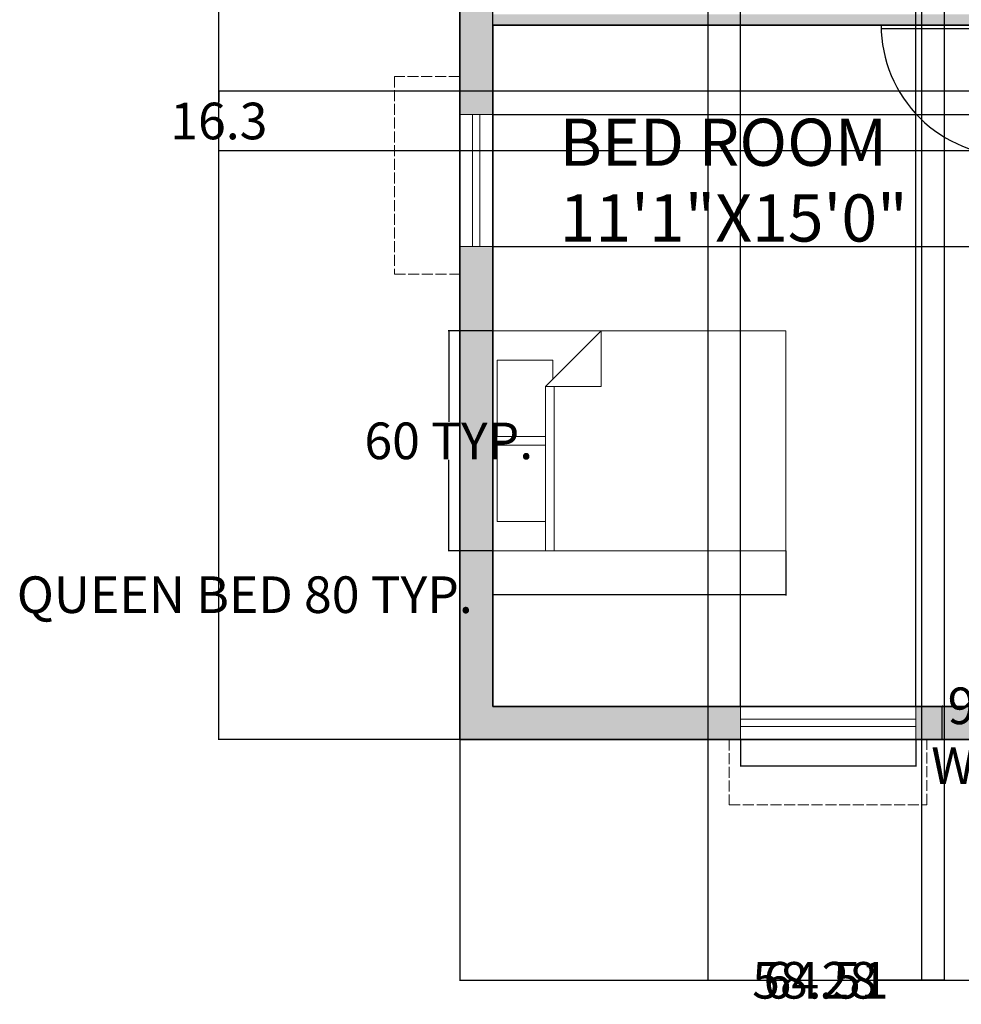
# Model space of a CAD drawing. Units: inches. Extents: x 300 to 1007, y 2 to 1069.
# Tile 1 of 12: x 300 to 557, y 2 to 271. Entities that reach past the tile are written whole.
import ezdxf

# ---------------------------------------------------------------- set-up
doc = ezdxf.new("R2010")
doc.units = ezdxf.units.IN
doc.header["$MEASUREMENT"] = 0
doc.linetypes.add('ACAD_ISO02W100', pattern=[15, 12, -3])
for name, color, linetype, lineweight in [('A-ANNO-DIMS', 2, 'Continuous', 18), ('A-AREA-IDEN', 7, 'Continuous', 18), ('A-DOOR', 3, 'Continuous', 25), ('A-FURN', 8, 'Continuous', 18), ('A-GLAZ', 4, 'Continuous', 18), ('A-GLAZ-OVHD', 8, 'ACAD_ISO02W100', 13), ('A-WALL', 7, 'Continuous', 35)]:
    doc.layers.add(name, color=color, linetype=linetype, lineweight=lineweight)
doc.layers.add('A-WALL-PATT', color=9, linetype='Continuous', lineweight=9, true_color=0xc7c8ca)
doc.styles.get("Standard").update_dxf_attribs({"font": 'arial.ttf'})
doc.dimstyles.get("Standard").update_dxf_attribs({"dimtxt": 10, "dimasz": 0.18, "dimexe": 0.18, "dimexo": 0.0625, "dimgap": 0.09, "dimtad": 0, "dimtih": 1, "dimtoh": 1, "dimdec": 0, "dimzin": 0, "dimdsep": 46, "dimlunit": 3, "dimtxsty": 'Standard', "dimcen": 0.09, "dimadec": 0, "dimazin": 0, "dimtfac": 1, "dimtdec": 0, "dimtofl": 0, "dimtmove": 0, "dimatfit": 3, "dimfxl": 1, "dimtolj": 1, "dimtzin": 0, "dimarcsym": 0})

# ---------------------------------------------------------------- blocks, each defined once
blk = doc.blocks.new('Bed - Queen')
for p, q in [((0, -80.00003), (0, 0)), ((0, 0), (59.99999, 0)), ((59.99999, 0), (59.99999, -80.00003)), ((7.99999, -1.2), (28.79998, -1.2)), ((7.99999, -14.4), (7.99999, -1.2)), ((28.79998, -1.2), (28.79998, -14.4)), ((31.19999, -1.2), (51.99999, -1.2)), ((31.19999, -14.4), (31.19999, -1.2)), ((51.99999, -1.2), (51.99999, -16.4)), ((0, -14.4), (44.8, -14.4)), ((59.99999, -29.6), (44.8, -14.4)), ((44.8, -14.4), (44.8, -29.6)), ((44.8, -16.8), (0, -16.8)), ((51.99999, -16.4), (46.79936, -16.4)), ((44.8, -29.6), (59.99999, -29.6)), ((59.99999, -80.00003), (0, -80.00003))]:
    blk.add_line(p, q)
blk = doc.blocks.new('WIN-48')
for p, q in [((-47.83, 0), (-47.83, 4.5)), ((-47.83, 4.5), (-47.83, -4.5)), ((0, 4.5), (0, -4.5)), ((0, 1), (-47.83, 1)), ((0, -1), (-47.83, -1))]:
    blk.add_line(p, q)
blk = doc.blocks.new('WIN-36')
for p, q in [((-36, -4.5), (-36, 4.5)), ((0, -4.5), (0, 4.5)), ((0, 1), (-36, 1)), ((-36, 0), (-36, -4.5)), ((0, -1), (-36, -1))]:
    blk.add_line(p, q)
blk = doc.blocks.new('WINDOW-HOOD-54')
at = {"ltscale": 0.25}
for p, q in [((0, 17.83), (-53.97, 17.83)), ((-53.97, 17.83), (-53.97, 0)), ((0, 0), (0, 17.83))]:
    blk.add_line(p, q, dxfattribs=at)
blk = doc.blocks.new('DOOR-SINGLE-36')
for p, q in [((-1, 0), (-1, 36)), ((0, 0), (0, 36))]:
    blk.add_line(p, q)
blk.add_arc((0, 0.34), 35.66, 90, 180.5503)
blk = doc.blocks.new('*D29')
at = {"layer": 'A-ANNO-DIMS', "color": 0, "lineweight": -2, "transparency": 16777216}
for p, q in [((429.12, 125.84), (429.12, 113.72)), ((509.12, 125.84), (509.12, 113.72)), ((429.12, 113.9), (428.94, 113.9)), ((508.94, 113.9), (429.3, 113.9))]:
    blk.add_line(p, q, dxfattribs=at)
at = {"layer": 'A-ANNO-DIMS', "color": 0, "transparency": 16777216}
for points in [[(429.3, 113.93), (429.3, 113.87), (429.12, 113.9)], [(508.94, 113.93), (508.94, 113.87), (509.12, 113.9)]]:
    blk.add_solid(points, dxfattribs=at)
at = {"layer": 'Defpoints', "color": 0, "transparency": 16777216}
for p in [(429.12, 125.9), (509.12, 125.9), (429.12, 113.9)]:
    blk.add_point(p, dxfattribs=at)
at = {"layer": 'A-ANNO-DIMS', "color": 0, "transparency": 16777216, "insert": (361.44, 113.9), "char_height": 10, "attachment_point": 5}
blk.add_mtext('\\A1;QUEEN BED 80 TYP.', dxfattribs=at)
blk = doc.blocks.new('*D30')
at = {"layer": 'A-ANNO-DIMS', "color": 0, "lineweight": -2, "transparency": 16777216}
for p, q in [((429.06, 185.9), (416.94, 185.9)), ((417.12, 185.72), (417.12, 161.09)), ((417.12, 126.08), (417.12, 150.7)), ((429.06, 125.9), (416.94, 125.9))]:
    blk.add_line(p, q, dxfattribs=at)
at = {"layer": 'A-ANNO-DIMS', "color": 0, "transparency": 16777216}
for points in [[(417.09, 185.72), (417.15, 185.72), (417.12, 185.9)], [(417.09, 126.08), (417.15, 126.08), (417.12, 125.9)]]:
    blk.add_solid(points, dxfattribs=at)
at = {"layer": 'Defpoints', "color": 0, "transparency": 16777216}
for p in [(417.12, 185.9), (429.12, 185.9), (429.12, 125.9)]:
    blk.add_point(p, dxfattribs=at)
at = {"layer": 'A-ANNO-DIMS', "color": 0, "transparency": 16777216, "insert": (417.12, 155.9), "char_height": 10, "attachment_point": 5}
blk.add_mtext('\\A1;60 TYP.', dxfattribs=at)
blk = doc.blocks.new('*D43')
at = {"layer": 'A-ANNO-DIMS', "color": 0, "lineweight": -2, "transparency": 16777216}
for p, q in [((496.77, 74.32), (496.77, 67.03)), ((544.6, 74.32), (544.6, 67.03)), ((496.95, 67.21), (544.42, 67.21)), ((544.6, 67.21), (544.78, 67.21))]:
    blk.add_line(p, q, dxfattribs=at)
at = {"layer": 'A-ANNO-DIMS', "color": 0, "transparency": 16777216}
for points in [[(496.95, 67.24), (496.95, 67.18), (496.77, 67.21)], [(544.42, 67.24), (544.42, 67.18), (544.6, 67.21)]]:
    blk.add_solid(points, dxfattribs=at)
at = {"layer": 'Defpoints', "color": 0, "transparency": 16777216}
for p in [(496.77, 74.38), (544.6, 74.38), (544.6, 67.21)]:
    blk.add_point(p, dxfattribs=at)
at = {"layer": 'A-ANNO-DIMS', "color": 0, "transparency": 16777216, "insert": (602, 67.21), "char_height": 10, "attachment_point": 5}
blk.add_mtext('\\A1;WINDOW 48 TYP.', dxfattribs=at)
blk = doc.blocks.new('*D44')
at = {"layer": 'A-ANNO-DIMS', "color": 0, "lineweight": -2, "transparency": 16777216}
for p, q in [((544.67, 83.38), (551.96, 83.38)), ((551.78, 83.38), (551.78, 83.56)), ((551.78, 83.56), (551.96, 83.56)), ((551.78, 74.56), (551.78, 83.2)), ((544.67, 74.38), (551.96, 74.38))]:
    blk.add_line(p, q, dxfattribs=at)
at = {"layer": 'A-ANNO-DIMS', "color": 0, "transparency": 16777216}
for points in [[(551.75, 83.2), (551.81, 83.2), (551.78, 83.38)], [(551.75, 74.56), (551.81, 74.56), (551.78, 74.38)]]:
    blk.add_solid(points, dxfattribs=at)
at = {"layer": 'Defpoints', "color": 0, "transparency": 16777216}
for p in [(544.6, 83.38), (551.78, 83.38), (544.6, 74.38)]:
    blk.add_point(p, dxfattribs=at)
at = {"layer": 'A-ANNO-DIMS', "color": 0, "transparency": 16777216, "insert": (572.5, 83.56), "char_height": 10, "attachment_point": 5}
blk.add_mtext('\\A1;9 TYP.', dxfattribs=at)
blk = doc.blocks.new('*D73')
at = {"layer": 'A-ANNO-DIMS', "color": 0, "lineweight": -2, "transparency": 16777216}
for p, q in [((420.12, 74.32), (420.12, 8.45)), ((910.12, 74.32), (910.12, 8.45)), ((420.3, 8.63), (653.8, 8.63)), ((909.94, 8.63), (676.44, 8.63))]:
    blk.add_line(p, q, dxfattribs=at)
at = {"layer": 'A-ANNO-DIMS', "color": 0, "transparency": 16777216}
for points in [[(420.3, 8.66), (420.3, 8.6), (420.12, 8.63)], [(909.94, 8.66), (909.94, 8.6), (910.12, 8.63)]]:
    blk.add_solid(points, dxfattribs=at)
at = {"layer": 'Defpoints', "color": 0, "transparency": 16777216}
for p in [(420.12, 74.38), (910.12, 74.38), (910.12, 8.63)]:
    blk.add_point(p, dxfattribs=at)
at = {"layer": 'A-ANNO-DIMS', "color": 0, "transparency": 16777216, "insert": (665.12, 8.63), "char_height": 10, "attachment_point": 5}
blk.add_mtext('\\A1;490', dxfattribs=at)
blk = doc.blocks.new('*D74')
at = {"layer": 'A-ANNO-DIMS', "color": 0, "lineweight": -2, "transparency": 16777216}
for p, q in [((478.76, 999.45), (354.19, 999.45)), ((354.37, 999.27), (354.37, 542.11)), ((354.37, 74.56), (354.37, 531.72)), ((420.06, 74.38), (354.19, 74.38))]:
    blk.add_line(p, q, dxfattribs=at)
at = {"layer": 'A-ANNO-DIMS', "color": 0, "transparency": 16777216}
for points in [[(354.34, 999.27), (354.4, 999.27), (354.37, 999.45)], [(354.34, 74.56), (354.4, 74.56), (354.37, 74.38)]]:
    blk.add_solid(points, dxfattribs=at)
at = {"layer": 'Defpoints', "color": 0, "transparency": 16777216}
for p in [(354.37, 999.45), (478.83, 999.45), (420.12, 74.38)]:
    blk.add_point(p, dxfattribs=at)
at = {"layer": 'A-ANNO-DIMS', "color": 0, "transparency": 16777216, "insert": (354.37, 536.92), "char_height": 10, "attachment_point": 5}
blk.add_mtext('\\A1;925', dxfattribs=at)
blk = doc.blocks.new('*D87')
at = {"layer": 'A-ANNO-DIMS', "color": 0, "lineweight": -2, "transparency": 16777216}
for p, q in [((805.89, 251.38), (354.19, 251.38)), ((354.37, 251.2), (354.37, 248.43)), ((354.37, 235.26), (354.37, 238.03)), ((805.89, 235.08), (354.19, 235.08))]:
    blk.add_line(p, q, dxfattribs=at)
at = {"layer": 'A-ANNO-DIMS', "color": 0, "transparency": 16777216}
for points in [[(354.34, 251.2), (354.4, 251.2), (354.37, 251.38)], [(354.34, 235.26), (354.4, 235.26), (354.37, 235.08)]]:
    blk.add_solid(points, dxfattribs=at)
at = {"layer": 'Defpoints', "color": 0, "transparency": 16777216}
for p in [(805.95, 251.38), (354.37, 235.08), (805.95, 235.08)]:
    blk.add_point(p, dxfattribs=at)
at = {"layer": 'A-ANNO-DIMS', "color": 0, "transparency": 16777216, "insert": (354.37, 243.23), "char_height": 10, "attachment_point": 5}
blk.add_mtext('\\A1;16.3', dxfattribs=at)
blk = doc.blocks.new('*D88')
at = {"layer": 'A-ANNO-DIMS', "color": 0, "lineweight": -2, "transparency": 16777216}
for p, q in [((429.12, 83.45), (429.12, 1063.03)), ((429.3, 1062.85), (445.92, 1062.85)), ((496.59, 1062.85), (479.97, 1062.85)), ((496.77, 83.45), (496.77, 1063.03))]:
    blk.add_line(p, q, dxfattribs=at)
at = {"layer": 'A-ANNO-DIMS', "color": 0, "transparency": 16777216}
for points in [[(429.3, 1062.88), (429.3, 1062.82), (429.12, 1062.85)], [(496.59, 1062.88), (496.59, 1062.82), (496.77, 1062.85)]]:
    blk.add_solid(points, dxfattribs=at)
at = {"layer": 'Defpoints', "color": 0, "transparency": 16777216}
for p in [(496.77, 1062.85), (429.12, 83.38), (496.77, 83.38)]:
    blk.add_point(p, dxfattribs=at)
at = {"layer": 'A-ANNO-DIMS', "color": 0, "transparency": 16777216, "insert": (462.95, 1062.85), "char_height": 10, "attachment_point": 5}
blk.add_mtext('\\A1;67.65', dxfattribs=at)
blk = doc.blocks.new('*D89')
at = {"layer": 'A-ANNO-DIMS', "color": 0, "lineweight": -2, "transparency": 16777216}
for p, q in [((544.6, 83.45), (544.6, 1063.03)), ((544.78, 1062.85), (554.56, 1062.85)), ((598.25, 1062.85), (588.48, 1062.85)), ((598.43, 83.45), (598.43, 1063.03))]:
    blk.add_line(p, q, dxfattribs=at)
at = {"layer": 'A-ANNO-DIMS', "color": 0, "transparency": 16777216}
for points in [[(544.78, 1062.88), (544.78, 1062.82), (544.6, 1062.85)], [(598.25, 1062.88), (598.25, 1062.82), (598.43, 1062.85)]]:
    blk.add_solid(points, dxfattribs=at)
at = {"layer": 'Defpoints', "color": 0, "transparency": 16777216}
for p in [(598.43, 1062.85), (544.6, 83.38), (598.43, 83.38)]:
    blk.add_point(p, dxfattribs=at)
at = {"layer": 'A-ANNO-DIMS', "color": 0, "transparency": 16777216, "insert": (571.52, 1062.85), "char_height": 10, "attachment_point": 5}
blk.add_mtext('\\A1;53.83', dxfattribs=at)
blk = doc.blocks.new('*D90')
at = {"layer": 'A-ANNO-DIMS', "color": 0, "lineweight": -2, "transparency": 16777216}
for p, q in [((429.18, 209), (974.48, 209)), ((974.3, 208.82), (974.3, 151.39)), ((974.3, 83.56), (974.3, 141)), ((429.18, 83.38), (974.48, 83.38))]:
    blk.add_line(p, q, dxfattribs=at)
at = {"layer": 'A-ANNO-DIMS', "color": 0, "transparency": 16777216}
for points in [[(974.27, 208.82), (974.33, 208.82), (974.3, 209)], [(974.27, 83.56), (974.33, 83.56), (974.3, 83.38)]]:
    blk.add_solid(points, dxfattribs=at)
at = {"layer": 'Defpoints', "color": 0, "transparency": 16777216}
for p in [(429.12, 209), (974.3, 209), (429.12, 83.38)]:
    blk.add_point(p, dxfattribs=at)
at = {"layer": 'A-ANNO-DIMS', "color": 0, "transparency": 16777216, "insert": (974.3, 146.19), "char_height": 10, "attachment_point": 5}
blk.add_mtext('\\A1;125.61', dxfattribs=at)
blk = doc.blocks.new('*D91')
at = {"layer": 'A-ANNO-DIMS', "color": 0, "lineweight": -2, "transparency": 16777216}
for p, q in [((429.18, 325.09), (974.48, 325.09)), ((974.3, 324.91), (974.3, 290.23)), ((974.3, 245.16), (974.3, 279.84)), ((429.18, 244.98), (974.48, 244.98))]:
    blk.add_line(p, q, dxfattribs=at)
at = {"layer": 'A-ANNO-DIMS', "color": 0, "transparency": 16777216}
for points in [[(974.27, 324.91), (974.33, 324.91), (974.3, 325.09)], [(974.27, 245.16), (974.33, 245.16), (974.3, 244.98)]]:
    blk.add_solid(points, dxfattribs=at)
at = {"layer": 'Defpoints', "color": 0, "transparency": 16777216}
for p in [(429.12, 325.09), (974.3, 325.09), (429.12, 244.98)]:
    blk.add_point(p, dxfattribs=at)
at = {"layer": 'A-ANNO-DIMS', "color": 0, "transparency": 16777216, "insert": (974.3, 285.04), "char_height": 10, "attachment_point": 5}
blk.add_mtext('\\A1;80.11', dxfattribs=at)
blk = doc.blocks.new('*D101')
at = {"layer": 'A-ANNO-DIMS', "color": 0, "lineweight": -2, "transparency": 16777216}
for p, q in [((487.83, 609.38), (487.83, 8.45)), ((552.34, 609.38), (552.34, 8.45)), ((488.01, 8.63), (504.06, 8.63)), ((552.16, 8.63), (536.11, 8.63))]:
    blk.add_line(p, q, dxfattribs=at)
at = {"layer": 'A-ANNO-DIMS', "color": 0, "transparency": 16777216}
for points in [[(488.01, 8.66), (488.01, 8.6), (487.83, 8.63)], [(552.16, 8.66), (552.16, 8.6), (552.34, 8.63)]]:
    blk.add_solid(points, dxfattribs=at)
at = {"layer": 'Defpoints', "color": 0, "transparency": 16777216}
for p in [(487.83, 609.45), (552.34, 609.45), (552.34, 8.63)]:
    blk.add_point(p, dxfattribs=at)
at = {"layer": 'A-ANNO-DIMS', "color": 0, "transparency": 16777216, "insert": (520.08, 8.63), "char_height": 10, "attachment_point": 5}
blk.add_mtext('\\A1;64.51', dxfattribs=at)
blk = doc.blocks.new('*D105')
at = {"layer": 'A-ANNO-DIMS', "color": 0, "lineweight": -2, "transparency": 16777216}
for p, q in [((487.83, 990.38), (487.83, 8.45)), ((546.1, 990.38), (546.1, 8.45)), ((488.01, 8.63), (499.99, 8.63)), ((545.92, 8.63), (533.94, 8.63))]:
    blk.add_line(p, q, dxfattribs=at)
at = {"layer": 'A-ANNO-DIMS', "color": 0, "transparency": 16777216}
for points in [[(488.01, 8.66), (488.01, 8.6), (487.83, 8.63)], [(545.92, 8.66), (545.92, 8.6), (546.1, 8.63)]]:
    blk.add_solid(points, dxfattribs=at)
at = {"layer": 'Defpoints', "color": 0, "transparency": 16777216}
for p in [(487.83, 990.45), (546.1, 990.45), (546.1, 8.63)]:
    blk.add_point(p, dxfattribs=at)
at = {"layer": 'A-ANNO-DIMS', "color": 0, "transparency": 16777216, "insert": (516.97, 8.63), "char_height": 10, "attachment_point": 5}
blk.add_mtext('\\A1;58.28', dxfattribs=at)

msp = doc.modelspace()

# ---------------------------------------------------------------- hatches: boundary and pattern name
at = {"layer": 'A-WALL-PATT'}
h = msp.add_hatch(color=256, dxfattribs=at)
h.dxf.hatch_style = 1
h.paths.add_polyline_path([(546.104, 999.4468), (478.8267, 999.4468), (478.8267, 869.2798, -0.06322715), (487.8267, 868.1328), (487.8267, 990.4468), (546.104, 990.4468)])
h.paths.add_polyline_path([(630.4852, 999.4468), (582.106, 999.4468), (582.106, 990.4468), (613.8267, 990.4468), (613.8267, 867.4468), (622.8267, 867.4468), (622.8267, 990.4468), (630.4852, 990.4468)])
h.paths.add_polyline_path([(702.0883, 999.4468), (650.4653, 999.4468), (650.4653, 990.4468), (682.8267, 990.4468), (682.8267, 960.0824, -0.02530575), (685.8267, 960.0478), (685.8267, 990.4468), (702.0883, 990.4468)])
h.paths.add_polyline_path([(850.8267, 999.4468), (737.5888, 999.4468), (737.5888, 990.4468), (841.8267, 990.4468), (841.8267, 950.5685), (850.8267, 950.5685)])
h.paths.add_polyline_path([(685.8267, 930.4465), (682.8267, 930.4465), (682.8267, 888.4468), (682.8267, 867.4468), (685.8267, 867.4468), (697.4169, 867.4468), (697.4169, 870.4468), (685.8267, 870.4468), (685.8267, 888.4468)])
h.paths.add_polyline_path([(682.8267, 931.4465), (654.3436, 931.4465, 0.00843109), (654.3267, 930.4465), (682.8267, 930.4465)])
h.paths.add_polyline_path([(685.8267, 931.4465), (682.8267, 931.4465), (682.8267, 930.4465), (685.8267, 930.4465)])
h.paths.add_polyline_path([(682.8267, 888.4468), (622.8267, 888.4468), (622.8267, 885.4468), (682.8267, 885.4468)])
h.paths.add_polyline_path([(850.8267, 870.4468), (850.8267, 914.7851), (841.8267, 914.7851), (841.8267, 870.4468), (732.7101, 870.4468, -0.02120595), (732.8267, 867.4468), (779.8267, 867.4468), (779.8267, 749.4468), (782.8267, 749.4468), (788.8267, 749.4468), (788.8267, 861.4468), (841.8267, 861.4468), (841.8267, 749.4468), (850.8267, 749.4468)])
h.paths.add_polyline_path([(622.8267, 810.4468), (487.8267, 810.4468), (487.8267, 833.2626), (478.8267, 833.2626), (478.8267, 609.4468), (478.8267, 482.3847), (487.8267, 482.3847), (487.8267, 801.4468), (620.8267, 801.4468), (622.8267, 801.4468)])
h.paths.add_polyline_path([(680.8267, 729.4468), (620.8267, 729.4468), (620.8267, 765.8246, -0.02111352), (617.8267, 766.0562), (617.8267, 698.7303), (620.8267, 698.7303), (620.8267, 726.4468), (680.8267, 726.4468)])
h.paths.add_polyline_path([(620.8267, 668.8122, -0.02498293), (617.8267, 668.6448), (617.8267, 618.4468), (600.3357, 618.4468), (600.3357, 609.4468), (652.9929, 609.4468), (652.9929, 618.4468), (620.8267, 618.4468)])
h.paths.add_polyline_path([(552.3393, 618.4468), (487.8267, 618.4468), (487.8267, 609.4468), (552.3393, 609.4468)], flags=17)
h.paths.add_polyline_path([(694.5763, 618.4468), (683.8267, 618.4468), (683.8267, 726.4468), (683.8267, 749.4468), (680.8267, 749.4468), (680.8267, 740.4468), (680.8267, 726.4468), (680.8267, 618.4468), (674.1573, 618.4468), (674.1573, 609.4468), (680.8267, 609.4468), (694.5763, 609.4468)])
h.paths.add_polyline_path([(850.8267, 642.8902), (841.8267, 642.8902), (841.8267, 618.4468), (782.8267, 618.4468), (782.8267, 708.0513, -0.02308839), (779.8267, 707.9092), (779.8267, 618.4468), (730.1068, 618.4468), (730.1068, 609.4468), (779.8267, 609.4468), (841.8267, 609.4468), (841.8267, 482.3847), (850.8267, 482.3847)])
h.paths.add_polyline_path([(850.8267, 749.4468), (841.8267, 749.4468), (841.8267, 705.9119), (850.8267, 705.9119)])
h.paths.add_polyline_path([(841.8267, 749.4468), (782.8267, 749.4468), (779.8267, 749.4468), (761.9959, 749.4468), (761.9959, 740.4468), (779.8267, 740.4468), (812.3267, 740.4468), (841.8267, 740.4468)])
h.paths.add_polyline_path([(669.1457, 482.3847), (604.489, 482.3847), (604.489, 473.3847), (631.1217, 473.3847), (631.1217, 436.0244, -0.02504709), (634.1217, 436.1748), (634.1217, 436.4367), (634.1217, 473.3847), (669.1457, 473.3847)], flags=17)
h.paths.add_polyline_path([(580.5305, 482.3847), (571.1217, 482.3847), (541.0813, 482.3847), (541.0813, 473.3847), (562.1217, 473.3847), (562.1217, 326.3847), (571.1217, 326.3847), (571.1217, 362.3847), (631.1217, 362.3847), (631.1217, 326.3847), (706.9024, 326.3847, -0.02105388), (706.9999, 329.3847), (634.1217, 329.3847), (634.1217, 365.3847), (634.1217, 406.1748), (631.1217, 406.1748), (631.1217, 365.3847), (571.1217, 365.3847), (571.1217, 473.3847), (580.5305, 473.3847)])
h.paths.add_polyline_path([(493.4756, 482.3847), (420.1217, 482.3847), (420.1217, 445.3134), (429.1217, 445.3134), (429.1217, 473.3847), (493.4756, 473.3847)])
h.paths.add_polyline_path([(786.2236, 482.3847), (716.7793, 482.3847), (716.7793, 473.3847), (766.1217, 473.3847), (766.1217, 329.3847), (742.5583, 329.3847), (742.5583, 326.3847), (766.1217, 326.3847), (766.1217, 316.0647), (769.1217, 316.0647), (769.1217, 326.3847), (769.1217, 473.3847), (786.2236, 473.3847)])
h.paths.add_polyline_path([(910.1217, 482.3847), (822.7166, 482.3847), (822.7166, 473.3847), (901.1217, 473.3847), (901.1217, 402.5393), (910.1217, 402.5393)])
h.paths.add_polyline_path([(910.1217, 366.1034), (901.1217, 366.1034), (901.1217, 329.3847), (814.1217, 329.3847), (814.1217, 312.5176), (817.1217, 312.5176), (817.1217, 326.3847), (901.1217, 326.3847), (901.1217, 293.0319), (910.1217, 293.0319), (910.1217, 326.3847)])
h.paths.add_polyline_path([(910.1217, 268.9355), (901.1217, 268.9355), (901.1217, 254.3847), (817.1217, 254.3847), (817.1217, 290.5411, -0.03396715), (814.1217, 290.3847), (814.1217, 254.3847), (775.1217, 254.3847), (775.1217, 281.5164), (769.1217, 281.5164), (769.1217, 292.1577), (766.1217, 292.1577), (766.1217, 254.3847), (766.1217, 220.1938), (775.5079, 220.1938), (775.5079, 251.3847), (817.1217, 251.3847), (901.1217, 251.3847), (901.1217, 152.3847), (819.0246, 152.3847, -0.02493798), (818.9117, 149.3847), (901.1217, 149.3847), (901.1217, 92.3847), (901.1217, 83.3847), (874.3528, 83.3847), (874.3528, 74.3847), (910.1217, 74.3847), (910.1217, 92.3847), (910.1217, 149.3847)])
h.paths.add_polyline_path([(429.1217, 325.0924), (420.1217, 325.0924), (420.1217, 263.3847), (420.1217, 244.9834), (429.1217, 244.9834), (429.1217, 269.3847), (571.1217, 269.3847), (571.1217, 272.3847), (562.1217, 272.3847), (429.1217, 272.3847)])
h.paths.add_polyline_path([(429.1217, 208.998), (420.1217, 208.998), (420.1217, 74.3847), (496.7704, 74.3847), (496.7704, 83.3847), (429.1217, 83.3847)])
h.paths.add_polyline_path([(598.4322, 83.3847), (571.1217, 83.3847), (571.1217, 122.1171), (562.1217, 122.1171), (562.1217, 83.3847), (544.6031, 83.3847), (544.6031, 74.3847), (598.4322, 74.3847)])
h.paths.add_polyline_path([(797.0822, 83.3847), (769.1217, 83.3847), (769.1217, 149.3847), (788.9123, 149.3847), (788.9123, 152.3847), (769.1217, 152.3847), (769.1217, 178.0167), (766.1217, 178.0167), (766.1217, 152.3847), (735.3598, 152.3847), (735.3598, 143.3847), (766.1217, 143.3847), (766.1217, 83.3847), (634.1217, 83.3847), (634.1217, 143.3847), (659.7326, 143.3847), (659.7326, 152.3847), (634.1217, 152.3847), (634.1217, 194.3847), (571.1217, 194.3847), (571.1217, 233.7289, -0.06379947), (562.1217, 234.7942), (562.1217, 163.4485), (567.7403, 163.4485), (567.7403, 152.3847), (571.1217, 152.3847), (571.1217, 191.3847), (631.1217, 191.3847), (631.1217, 83.3847), (621.979, 83.3847), (621.979, 74.3847), (631.1217, 74.3847), (797.0822, 74.3847)])

# ---------------------------------------------------------------- linework, layer by layer
at = {"layer": 'A-WALL'}
for p, q in [((429.1217, 269.3847), (429.1217, 83.3847)), ((429.1217, 269.3847), (571.1217, 269.3847)), ((420.1217, 263.3847), (420.1217, 74.3847)), ((429.1217, 83.3847), (562.1217, 83.3847)), ((420.1217, 74.3847), (910.1217, 74.3847))]:
    msp.add_line(p, q, dxfattribs=at)
msp.add_lwpolyline([(571.1217, 482.3847), (420.1217, 482.3847), (420.1217, 263.3847)], dxfattribs=at)

# ---------------------------------------------------------------- block references
at = {"layer": 'A-DOOR', "rotation": 90.00000000000108}
msp.add_blockref('DOOR-SINGLE-36', (571.1217, 269.3847), dxfattribs=at)
at = {"layer": 'A-FURN', "rotation": 89.99999999999999}
msp.add_blockref('Bed - Queen', (429.1217, 125.8991), dxfattribs=at)
at = {"layer": 'A-GLAZ', "xscale": 0.9995380606049479, "rotation": 90}
msp.add_blockref('WIN-36', (424.6217, 244.9834), dxfattribs=at)
at = {"layer": 'A-GLAZ'}
msp.add_blockref('WIN-48', (544.6031, 78.8847), dxfattribs=at)
at = {"layer": 'A-GLAZ-OVHD'}
for p, rotation in [((420.1217, 255.3971), 90.00000000000007), ((493.6546, 74.3847), 180)]:
    msp.add_blockref('WINDOW-HOOD-54', p, dxfattribs=dict(at, rotation=rotation))

# ---------------------------------------------------------------- texts
at = {"layer": 'A-AREA-IDEN'}
for s, height, p in [('BED ROOM', 12.87594, (447.3715, 230.9895)), ('11\'1"X15\'0"', 12.875935, (447.3715, 210.3054))]:
    msp.add_text(s, height=height, dxfattribs=at).set_placement(p)

# ---------------------------------------------------------------- dimensions: what is measured, and where the dimension line sits
at = {"layer": 'A-ANNO-DIMS'}
for base, p1, p2, override, picture, middle in [((496.7704, 1062.8469), (429.1217, 83.3847), (496.7704, 83.3847), {"dimdec": 2, "dimlfac": 1, "dimrnd": 0, "dimzin": 0, "dimdsep": 46, "dimlunit": 2}, '*D88', (462.946, 1062.8469)), ((598.4322, 1062.8469), (544.6031, 83.3847), (598.4322, 83.3847), {"dimdec": 2, "dimlfac": 1, "dimrnd": 0, "dimzin": 0, "dimdsep": 46, "dimlunit": 2}, '*D89', (571.5176, 1062.8469)), ((546.104, 8.6288), (487.8267, 990.4468), (546.104, 990.4468), {"dimdec": 2, "dimlfac": 1, "dimrnd": 0, "dimzin": 0, "dimdsep": 46, "dimlunit": 2}, '*D105', (516.9653, 8.6288)), ((552.3393, 8.6288), (487.8267, 609.4468), (552.3393, 609.4468), {"dimdec": 2, "dimlfac": 1, "dimrnd": 0, "dimzin": 0, "dimdsep": 46, "dimlunit": 2}, '*D101', (520.083, 8.6288)), ((910.1217, 8.6288), (420.1217, 74.3847), (910.1217, 74.3847), {"dimdec": 0, "dimlfac": 1, "dimrnd": 0, "dimzin": 0, "dimdsep": 46, "dimlunit": 2}, '*D73', (665.1217, 8.6288))]:
    dim = msp.add_linear_dim(base=base, p1=p1, p2=p2, dimstyle='Standard', override=override, dxfattribs=at)
    dim.commit()
    dim.dimension.update_dxf_attribs({"geometry": picture, "text_midpoint": middle})
for base, p1, p2, override, picture, middle in [((354.3658, 999.4468), (420.1217, 74.3847), (478.8267, 999.4468), {"dimdec": 0, "dimlfac": 1, "dimrnd": 0, "dimzin": 0, "dimdsep": 46, "dimlunit": 2}, '*D74', (354.3658, 536.9158)), ((974.3023, 325.0924), (429.1217, 244.9834), (429.1217, 325.0924), {"dimdec": 2, "dimlfac": 1, "dimrnd": 0, "dimzin": 0, "dimdsep": 46, "dimlunit": 2}, '*D91', (974.3023, 285.0379)), ((354.3658, 235.0834), (805.95, 251.3847), (805.95, 235.0834), {"dimdec": 1, "dimlfac": 1, "dimrnd": 0, "dimzin": 0, "dimdsep": 46, "dimlunit": 2}, '*D87', (354.3658, 243.2341)), ((974.3023, 208.998), (429.1217, 83.3847), (429.1217, 208.998), {"dimdec": 2, "dimlfac": 1, "dimrnd": 0, "dimzin": 0, "dimdsep": 46, "dimlunit": 2}, '*D90', (974.3023, 146.1913))]:
    dim = msp.add_linear_dim(base=base, p1=p1, p2=p2, angle=90, dimstyle='Standard', override=override, dxfattribs=at)
    dim.commit()
    dim.dimension.update_dxf_attribs({"geometry": picture, "text_midpoint": middle})
for base, p1, p2, angle, text, picture, middle in [((417.1217, 185.8991), (429.1217, 125.8991), (429.1217, 185.8991), 90, '<> TYP.', '*D30', (417.1217, 155.8991)), ((429.1217, 113.8991), (509.1217, 125.8991), (429.1217, 125.8991), 180, 'QUEEN BED <> TYP.', '*D29', (361.4404, 113.8991)), ((551.778, 83.3847), (544.6031, 74.3847), (544.6031, 83.3847), 90, '<> TYP.', '*D44', (572.5016, 83.5647))]:
    dim = msp.add_linear_dim(base=base, p1=p1, p2=p2, angle=angle, text=text, dimstyle='Standard', override={"dimdec": 0, "dimlfac": 1, "dimrnd": 0, "dimzin": 0, "dimdsep": 46, "dimlunit": 2}, dxfattribs=at)
    dim.commit()
    dim.dimension.update_dxf_attribs({"geometry": picture, "text_midpoint": middle})
dim = msp.add_linear_dim(base=(544.6031, 67.2098), p1=(496.7704, 74.3847), p2=(544.6031, 74.3847), text='WINDOW <> TYP.', dimstyle='Standard', override={"dimdec": 0, "dimlfac": 1, "dimrnd": 0, "dimzin": 0, "dimdsep": 46, "dimlunit": 2}, dxfattribs=at)
dim.commit()
dim.dimension.update_dxf_attribs({"geometry": '*D43', "text_midpoint": (602.0047, 67.2098)})

doc.saveas('drawing.dxf')
